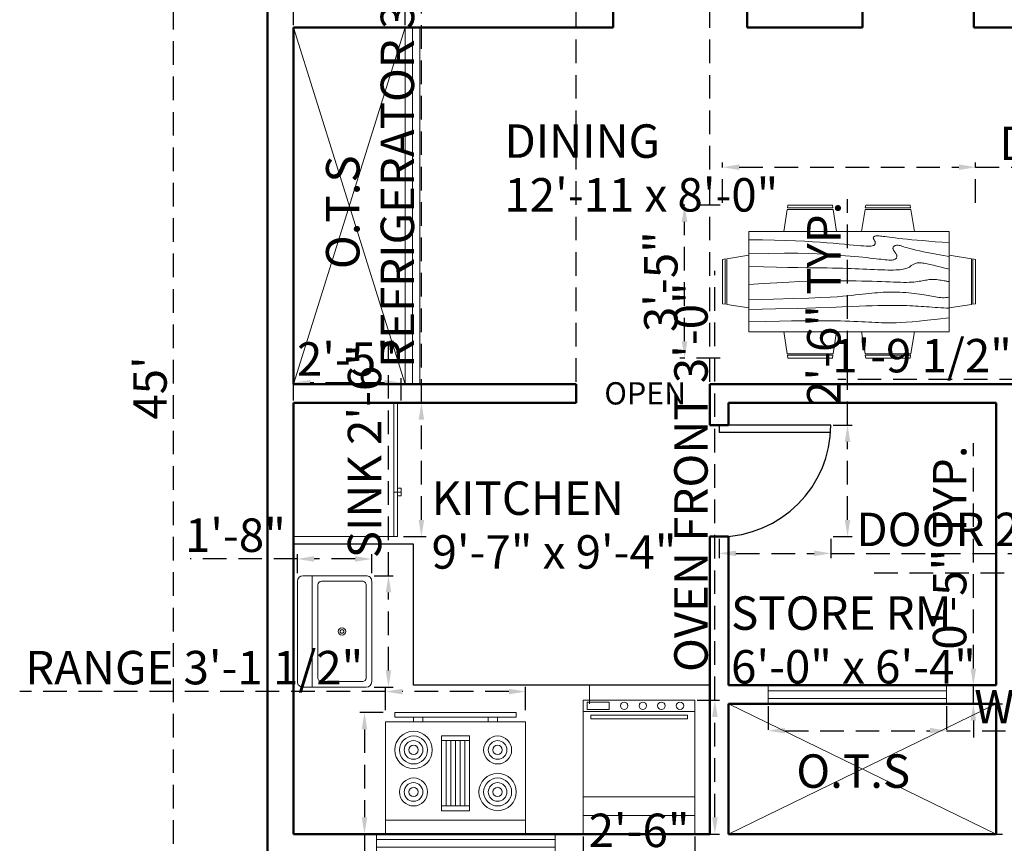
# Model space of a CAD drawing. Units: inches. Extents: x 3209 to 7144, y 1281 to 3076.
# Tile 2 of 5: x 3209 to 3474, y 1459 to 1680. Entities that reach past the tile are written whole.
import ezdxf

# ---------------------------------------------------------------- set-up
doc = ezdxf.new("R2010")
doc.units = ezdxf.units.IN
doc.linetypes.add('HIDDEN', pattern=[9.525, 6.35, -3.175])
for name, color, linetype, lineweight in [('A-ANNO-DIMS', 244, 'HIDDEN', 18), ('A-ANNO-TEXT', 7, 'Continuous', 18), ('A-AREA-IDEN', 7, 'Continuous', 25), ('A-DOOR', 4, 'Continuous', 25), ('A-EQPM', 9, 'Continuous', 18), ('A-FLOR-CASE', 8, 'Continuous', 25), ('A-FLOR-FIXT', 9, 'Continuous', 18), ('A-FLOR-OPEN', 8, 'Continuous', 13), ('A-FURN', 8, 'Continuous', 18), ('A-GLAZ', 4, 'Continuous', 18), ('A-WALL', 7, 'Continuous', 50)]:
    doc.layers.add(name, color=color, linetype=linetype, lineweight=lineweight)
doc.styles.get("Standard").update_dxf_attribs({"font": 'arial.ttf'})
doc.dimstyles.new('ISO-25', dxfattribs={"dimtxt": 9, "dimasz": 4.5, "dimexe": 1.25, "dimexo": 0.625, "dimtad": 1, "dimdec": 0, "dimlunit": 3, "dimtxsty": 'Standard', "dimcen": 2.5, "dimadec": 0, "dimazin": 0, "dimtfac": 1, "dimtdec": 0, "dimtmove": 0, "dimatfit": 3, "dimfxl": 1, "dimarcsym": 0})

# ---------------------------------------------------------------- blocks, each defined once
blk = doc.blocks.new('Dining Set - 36 x 72 in.')
for p, q in [((-22.2343, 26.00059), (-23.4847, 17.99762)), ((-22.2304, 26), (-5.7608, 26)), ((-22, 27.5), (-22.1562, 26.50042)), ((-5.8416, 26.5), (-22.1534, 26.5)), ((-22, 27.5), (-6, 27.5)), ((-5.8437, 26.49966), (-6, 27.5)), ((-4.5152, 17.99762), (-5.7655, 25.99926)), ((5.7657, 26.00059), (4.5153, 17.99762)), ((5.7696, 26), (22.2392, 26)), ((6, 27.5), (5.8438, 26.50042)), ((22.1584, 26.5), (5.8466, 26.5)), ((6, 27.5), (22, 27.5)), ((22.1563, 26.49966), (22, 27.5)), ((23.4848, 17.99762), (22.2345, 25.99926)), ((36, 18), (-36, 18)), ((-36, 18), (-36, -18)), ((36, -18), (36, 18)), ((-45.5, 8), (-44.5004, 8.15617)), ((-45.5, 8), (-45.5, -8)), ((-44.5, -8.15843), (-44.5, 8.15338)), ((-44.0006, 8.23428), (-35.9976, 9.48474)), ((-44, 8.23041), (-44, -8.23915)), ((44.0006, 8.23428), (35.9976, 9.48474)), ((44, 8.23041), (44, -8.23915)), ((44.5, -8.15843), (44.5, 8.15338)), ((45.5, 8), (44.5005, 8.15617)), ((45.5, 8), (45.5, -8)), ((-44.4997, -8.15631), (-45.5, -8)), ((-35.9976, -9.48476), (-43.9993, -8.2345)), ((35.9976, -9.48476), (43.9993, -8.2345)), ((44.4997, -8.15631), (45.5, -8)), ((-36, -18), (36, -18)), ((-22.2343, -26.0006), (-23.4847, -17.99762)), ((-4.5152, -17.99762), (-5.7655, -25.99928)), ((5.7657, -26.0006), (4.5153, -17.99762)), ((23.4848, -17.99762), (22.2345, -25.99928)), ((-22.2304, -26), (-5.7608, -26)), ((-22, -27.5), (-22.1562, -26.50044)), ((-5.8416, -26.5), (-22.1534, -26.5)), ((-22, -27.5), (-6, -27.5)), ((-5.8437, -26.49967), (-6, -27.5)), ((5.7696, -26), (22.2392, -26)), ((6, -27.5), (5.8438, -26.50044)), ((22.1584, -26.5), (5.8466, -26.5)), ((6, -27.5), (22, -27.5)), ((22.1563, -26.49967), (22, -27.5))]:
    blk.add_line(p, q)
for points in [[(-36, 15), (-31.1772, 14.97754), (-26.8079, 14.91406), (-22.8538, 14.81543), (-19.276, 14.6875), (-16.0362, 14.53613), (-13.0957, 14.36718), (-10.4159, 14.18652), (-7.9583, 14), (-5.6904, 13.81315), (-3.6035, 13.63021), (-1.6954, 13.45508), (0.0365, 13.29166), (1.5945, 13.14388), (2.9811, 13.01562), (4.1988, 12.9108), (5.25, 12.83333), (6.1393, 12.78613), (6.8802, 12.76823), (7.4883, 12.77767), (7.9792, 12.8125), (8.3685, 12.87077), (8.6719, 12.95052), (8.9049, 13.0498), (9.0833, 13.16666), (9.2205, 13.29899), (9.3216, 13.44401), (9.3895, 13.59879), (9.4271, 13.76041), (9.4373, 13.92594), (9.4232, 14.09245), (9.3875, 14.257), (9.3333, 14.41666), (9.2638, 14.56917), (9.1836, 14.71484), (9.0975, 14.85465), (9.0104, 14.98958), (8.9272, 15.1206), (8.8529, 15.2487), (8.7922, 15.37483), (8.75, 15.5), (8.7305, 15.62467), (8.7344, 15.74739), (8.7617, 15.86621), (8.8125, 15.97916), (8.8867, 16.08431), (8.9844, 16.17968), (9.1055, 16.26334), (9.25, 16.33333), (9.4189, 16.38802), (9.6172, 16.42708), (9.8506, 16.45052), (10.125, 16.45833), (10.4463, 16.45052), (10.8203, 16.42708), (11.2529, 16.38802), (11.75, 16.33333), (12.3184, 16.26318), (12.9694, 16.17838), (13.7151, 16.07991), (14.5677, 15.96875), (15.5395, 15.84586), (16.6426, 15.71224), (17.8893, 15.56884), (19.2917, 15.41666), (20.859, 15.25667), (22.5879, 15.08984), (24.4721, 14.91715), (26.5052, 14.73958), (28.6809, 14.5581), (30.9929, 14.3737), (33.4347, 14.18733), (36, 14)], [(-36, 10), (-28.9766, 10.14274), (-23.1725, 10.20442), (-18.4241, 10.19775), (-14.5677, 10.13541), (-11.4399, 10.03011), (-8.877, 9.89453), (-6.7154, 9.74137), (-4.7917, 9.58333), (-2.9698, 9.43082), (-1.2246, 9.28515), (0.4415, 9.14534), (2.026, 9.01041), (3.5266, 8.87939), (4.9408, 8.7513), (6.266, 8.62516), (7.5, 8.5), (8.6411, 8.37549), (9.6914, 8.2539), (10.6538, 8.13818), (11.5312, 8.03125), (12.3267, 7.93603), (13.043, 7.85547), (13.6831, 7.79248), (14.25, 7.75), (14.7471, 7.7303), (15.1797, 7.73307), (15.5537, 7.75732), (15.875, 7.80208), (16.1494, 7.86637), (16.3828, 7.94922), (16.5811, 8.04964), (16.75, 8.16666), (16.8944, 8.29915), (17.0143, 8.44531), (17.1089, 8.60319), (17.1771, 8.77083), (17.218, 8.94629), (17.2305, 9.1276), (17.2137, 9.31282), (17.1667, 9.5), (17.0895, 9.6875), (16.987, 9.875), (16.8649, 10.0625), (16.7292, 10.25), (16.5856, 10.4375), (16.4401, 10.625), (16.2985, 10.8125), (16.1667, 11), (16.05, 11.18733), (15.9518, 11.3737), (15.8752, 11.5581), (15.8229, 11.73958), (15.798, 11.91715), (15.8034, 12.08984), (15.842, 12.25667), (15.9167, 12.41666), (16.0295, 12.56836), (16.1784, 12.70833), (16.3605, 12.83268), (16.5729, 12.9375), (16.8127, 13.01888), (17.0768, 13.07291), (17.3625, 13.0957), (17.6667, 13.08333), (17.9894, 13.03312), (18.3418, 12.94726), (18.7382, 12.82918), (19.1927, 12.68229), (19.7195, 12.51001), (20.3327, 12.31575), (21.0465, 12.10294), (21.875, 11.875), (22.8357, 11.63354), (23.959, 11.37304), (25.2786, 11.08618), (26.8282, 10.76562), (28.6414, 10.40405), (30.752, 9.99414), (33.1936, 9.52856), (36, 9)], [(-36, 5.5), (-30.7157, 5.3348), (-26.069, 5.20963), (-21.9946, 5.11767), (-18.4271, 5.05208), (-15.3009, 5.00602), (-12.5508, 4.97265), (-10.1112, 4.94515), (-7.9167, 4.91666), (-5.909, 4.88167), (-4.0586, 4.83984), (-2.3429, 4.79215), (-0.7396, 4.73958), (0.7739, 4.6831), (2.22, 4.6237), (3.6213, 4.56233), (5, 4.5), (6.373, 4.43782), (7.7344, 4.3776), (9.0723, 4.32129), (10.375, 4.27083), (11.6309, 4.22819), (12.8281, 4.19531), (13.9551, 4.17415), (15, 4.16666), (15.954, 4.17448), (16.819, 4.19791), (17.6001, 4.23698), (18.3021, 4.29166), (18.9299, 4.36198), (19.4883, 4.44791), (19.9823, 4.54948), (20.4167, 4.66666), (20.7969, 4.79899), (21.1302, 4.94401), (21.4245, 5.09879), (21.6875, 5.26041), (21.9271, 5.42594), (22.1511, 5.59245), (22.3672, 5.757), (22.5834, 5.91666), (22.8065, 6.06868), (23.0404, 6.21093), (23.2879, 6.34147), (23.5521, 6.45833), (23.8358, 6.55957), (24.142, 6.64323), (24.4735, 6.70735), (24.8334, 6.75), (25.2235, 6.76969), (25.642, 6.76692), (26.0858, 6.74267), (26.5521, 6.69791), (27.0379, 6.63362), (27.5404, 6.55078), (28.0565, 6.45036), (28.5834, 6.33333), (29.1242, 6.19987), (29.7071, 6.04687), (30.3661, 5.87044), (31.1354, 5.66666), (32.0493, 5.43164), (33.142, 5.16146), (34.4475, 4.85221), (36, 4.5)], [(-36, -1), (-30.7915, -0.6591), (-26.0195, -0.38216), (-21.6519, -0.16284), (-17.6563, 0.00521), (-14.0005, 0.12833), (-10.6523, 0.21289), (-7.5796, 0.26522), (-4.75, 0.29166), (-2.134, 0.29793), (0.2878, 0.28711), (2.5317, 0.26163), (4.6146, 0.22396), (6.5529, 0.17651), (8.3633, 0.12174), (10.0623, 0.06209), (11.6667, 0), (13.1899, -0.06201), (14.6341, -0.1211), (15.9982, -0.17432), (17.2813, -0.21875), (18.4823, -0.25147), (19.6003, -0.26953), (20.6343, -0.27002), (21.5834, -0.25), (22.4481, -0.20768), (23.2357, -0.14584), (23.9549, -0.06836), (24.6146, 0.02083), (25.2235, 0.11784), (25.7904, 0.21875), (26.3241, 0.31966), (26.8334, 0.41666), (27.3265, 0.50618), (27.8099, 0.58593), (28.2894, 0.65397), (28.7709, 0.70833), (29.2601, 0.74707), (29.763, 0.76823), (30.2855, 0.76985), (30.8334, 0.75), (31.4088, 0.70784), (31.9994, 0.64713), (32.589, 0.57275), (33.1615, 0.48958), (33.7008, 0.4025), (34.1908, 0.3164), (34.6153, 0.23616), (34.9584, 0.16666), (35.2099, 0.11165), (35.3848, 0.07031), (35.504, 0.04069), (35.5886, 0.02083), (35.6594, 0.00879), (35.7377, 0.0026), (35.8442, 0.00032), (36, 0)], [(-36, -6.5), (-27.1843, -6.31267), (-20.084, -6.1263), (-14.469, -5.9419), (-10.1094, -5.76042), (-6.7752, -5.58285), (-4.2363, -5.41016), (-2.2629, -5.24333), (-0.625, -5.08334), (0.8708, -4.93099), (2.2715, -4.78646), (3.5872, -4.64974), (4.8281, -4.52084), (6.0046, -4.39974), (7.127, -4.28646), (8.2053, -4.18099), (9.25, -4.08334), (10.2705, -3.99382), (11.2734, -3.91407), (12.2647, -3.84603), (13.25, -3.79167), (14.2354, -3.75293), (15.2266, -3.73177), (16.2295, -3.73015), (17.25, -3.75), (18.2912, -3.79248), (19.3451, -3.85547), (20.4009, -3.93604), (21.4479, -4.03125), (22.4754, -4.13819), (23.4727, -4.25391), (24.4289, -4.37549), (25.3334, -4.5), (26.1785, -4.62492), (26.9694, -4.74935), (27.7145, -4.87281), (28.4219, -4.99479), (29.1, -5.11483), (29.7572, -5.23242), (30.4016, -5.34709), (31.0417, -5.45834), (31.6837, -5.56437), (32.3262, -5.65821), (32.9658, -5.73153), (33.599, -5.77604), (34.2224, -5.78345), (34.8327, -5.74545), (35.4264, -5.65373), (36, -5.5)], [(-36, -10), (-26.4022, -9.81299), (-18.4675, -9.62891), (-11.9839, -9.45069), (-6.7396, -9.28125), (-2.5226, -9.12354), (0.8789, -8.98047), (3.6769, -8.85498), (6.0833, -8.75), (8.2767, -8.66765), (10.3021, -8.60677), (12.1712, -8.56543), (13.8958, -8.54167), (15.4876, -8.53353), (16.9583, -8.53907), (18.3197, -8.55632), (19.5834, -8.58334), (20.7616, -8.61841), (21.8685, -8.66081), (22.9188, -8.71004), (23.9271, -8.76563), (24.9081, -8.82707), (25.8763, -8.89388), (26.8465, -8.96558), (27.8334, -9.04167), (28.8474, -9.12118), (29.8828, -9.20117), (30.93, -9.27824), (31.9792, -9.34896), (33.0205, -9.40991), (34.0443, -9.45768), (35.0407, -9.48885), (36, -9.5)], [(-36, -14.5), (-30.0881, -14.33513), (-25.0332, -14.21224), (-20.7312, -14.12647), (-17.0781, -14.07292), (-13.97, -14.04671), (-11.3027, -14.04297), (-8.9724, -14.05681), (-6.875, -14.08334), (-4.9224, -14.11833), (-3.0905, -14.16016), (-1.3709, -14.20785), (0.2448, -14.26042), (1.7647, -14.3169), (3.1973, -14.3763), (4.5507, -14.43767), (5.8333, -14.5), (7.0554, -14.5621), (8.235, -14.62175), (9.3922, -14.67652), (10.5469, -14.72396), (11.7192, -14.76164), (12.929, -14.78711), (14.1965, -14.79794), (15.5417, -14.79167), (16.9933, -14.76424), (18.6152, -14.70508), (20.4804, -14.60197), (22.6615, -14.44271), (25.2312, -14.21509), (28.2624, -13.9069), (31.8277, -13.50594), (36, -13)]]:
    blk.add_lwpolyline(points)
blk = doc.blocks.new('Range-Oven - 30 in front')
for p, q in [((0, 33.00005), (30, 33.00005)), ((30, 10), (0, 10)), ((0, 5), (30, 5))]:
    blk.add_line(p, q)
for points in [[(0, 0), (0, 36.00005), (30, 36.00005), (30, 0)], [(1, 33.50005), (1, 35.50005), (7, 35.50005), (7, 33.50005)], [(2, 31.00005), (2, 32.00005), (28, 32.00005), (28, 31.00005)]]:
    blk.add_lwpolyline(points, close=True)
for centre in [(11, 34.50005), (16, 34.50005), (21, 34.50005), (26, 34.50005)]:
    blk.add_circle(centre, 1)
blk = doc.blocks.new('Sink-single - 30 in top')
blk.add_line((-15, -3.999996), (15, -3.999996))
for points in [[(-13.5, 0), (13.5, 0)], [(-15, -18.499996), (-15, -1.5)], [(15, -1.5), (15, -18.499996)], [(-13.5, -17.499996), (-13.5, -6.499996)], [(-12.5, -5.499996), (12.5, -5.499996)], [(13.5, -6.499996), (13.5, -17.499996)], [(12.5, -18.499996), (-12.5, -18.499996)], [(13.5, -19.999996), (-13.5, -19.999996)]]:
    blk.add_lwpolyline(points)
for radius in [1, 0.5]:
    blk.add_circle((0, -11.999996), radius)
for centre, radius, start, end in [((-13.5, -1.5), 1.5, 90, 180), ((13.5, -1.5), 1.5, 0, 90), ((-12.5, -6.499996), 1, 90, 180), ((12.5, -6.499996), 1, 0, 90), ((-13.5, -18.499996), 1.5, 180, 270), ((-12.5, -17.499996), 1, 180, 270), ((12.5, -17.499996), 1, 270, 0), ((13.5, -18.499996), 1.5, 270, 0)]:
    blk.add_arc(centre, radius, start, end)
blk = doc.blocks.new('Refrigerator-2 door - 36 in top')
for p, q in [((0, -26.999999), (36, -26.999999)), ((11, -27.999999), (11, -28.999999)), ((11, -28.999999), (13, -28.999999)), ((12, -26.999999), (12, -28.999999)), ((13, -28.999999), (13, -27.999999))]:
    blk.add_line(p, q)
blk.add_lwpolyline([(0, -27.999999), (0, 0), (36, 0), (36, -27.999999)], close=True)
blk = doc.blocks.new('Range-Oven - 30 in top')
for p, q in [((0, -3), (30, -3)), ((12, -6), (18, -6)), ((13, -20), (13, -6)), ((14, -6), (14, -20)), ((15, -20), (15, -6)), ((16, -6), (16, -20)), ((17, -20), (17, -6)), ((18, -20), (12, -20)), ((6, -24), (6, -25)), ((8, -25), (8, -24)), ((22, -25), (22, -24)), ((24, -24), (24, -25))]:
    blk.add_line(p, q)
for points in [[(0, -24), (0, 0), (30, 0), (30, -24)], [(12, -21), (12, -5), (18, -5), (18, -21)], [(2, -26), (2, -25), (28, -25), (28, -26)]]:
    blk.add_lwpolyline(points, close=True)
for centre, radius in [((6, -9), 4), ((6, -9), 3), ((24, -9), 3), ((6, -9), 2), ((6, -9), 1), ((24, -9), 2), ((24, -9), 1), ((24, -18), 4), ((6, -18), 3), ((6, -18), 2), ((24, -18), 3), ((24, -18), 2), ((6, -18), 1), ((24, -18), 1)]:
    blk.add_circle(centre, radius)
blk = doc.blocks.new('*D15')
at = {"layer": 'A-ANNO-DIMS', "color": 0, "lineweight": -2, "transparency": 16777216}
for p, q in [((3275.31, 1851.27), (3249.46, 1851.27)), ((3250.71, 1315.77), (3250.71, 1846.77)), ((3275.31, 1311.27), (3249.46, 1311.27))]:
    blk.add_line(p, q, dxfattribs=at)
at = {"layer": 'A-ANNO-DIMS', "color": 0, "transparency": 16777216}
for points in [[(3249.96, 1846.77), (3251.46, 1846.77), (3250.71, 1851.27)], [(3249.96, 1315.77), (3251.46, 1315.77), (3250.71, 1311.27)]]:
    blk.add_solid(points, dxfattribs=at)
at = {"layer": 'Defpoints', "color": 0, "transparency": 16777216}
for p in [(3250.71, 1851.27), (3275.94, 1851.27), (3275.94, 1311.27)]:
    blk.add_point(p, dxfattribs=at)
at = {"layer": 'A-ANNO-DIMS', "color": 0, "transparency": 16777216, "insert": (3245.51, 1581.27), "char_height": 9, "attachment_point": 5, "rotation": 90}
blk.add_mtext("45'", dxfattribs=at)
blk = doc.blocks.new('DOOR-SWING-30IN')
for p, q in [((30, 30), (0, 30)), ((0, 30), (0, 28)), ((30, 28), (0, 28))]:
    blk.add_line(p, q)
blk.add_arc((0, 30), 30, 270, 0)
blk = doc.blocks.new('WINDOW-48IN-WALL5')
for p, q in [((0, 5), (0, 0)), ((0, 3.5), (48, 3.5)), ((48, 5), (48, 0)), ((0, 1.5), (48, 1.5))]:
    blk.add_line(p, q)
blk = doc.blocks.new('*D42')
at = {"layer": 'A-ANNO-DIMS', "color": 0, "lineweight": -2, "transparency": 16777216}
for p, q in [((3397.44, 1540.64), (3397.44, 1535.52)), ((3427.44, 1540.64), (3427.44, 1535.52)), ((3401.94, 1536.77), (3422.94, 1536.77)), ((3427.44, 1536.77), (3528.81, 1536.77))]:
    blk.add_line(p, q, dxfattribs=at)
at = {"layer": 'A-ANNO-DIMS', "color": 0, "transparency": 16777216}
for points in [[(3401.94, 1537.52), (3401.94, 1536.02), (3397.44, 1536.77)], [(3422.94, 1537.52), (3422.94, 1536.02), (3427.44, 1536.77)]]:
    blk.add_solid(points, dxfattribs=at)
at = {"layer": 'Defpoints', "color": 0, "transparency": 16777216}
for p in [(3397.44, 1541.27), (3427.44, 1541.27), (3427.44, 1536.77)]:
    blk.add_point(p, dxfattribs=at)
at = {"layer": 'A-ANNO-DIMS', "color": 0, "transparency": 16777216, "insert": (3480.37, 1542.05), "char_height": 9, "attachment_point": 5}
blk.add_mtext('DOOR 2\'-6" TYP.', dxfattribs=at)
blk = doc.blocks.new('*D43')
at = {"layer": 'A-ANNO-DIMS', "color": 0, "lineweight": -2, "transparency": 16777216}
for p, q in [((3431.94, 1571.27), (3431.94, 1632.03)), ((3428.06, 1571.27), (3433.19, 1571.27)), ((3431.94, 1545.77), (3431.94, 1566.77)), ((3428.06, 1541.27), (3433.19, 1541.27))]:
    blk.add_line(p, q, dxfattribs=at)
at = {"layer": 'A-ANNO-DIMS', "color": 0, "transparency": 16777216}
for points in [[(3431.19, 1566.77), (3432.69, 1566.77), (3431.94, 1571.27)], [(3431.19, 1545.77), (3432.69, 1545.77), (3431.94, 1541.27)]]:
    blk.add_solid(points, dxfattribs=at)
at = {"layer": 'Defpoints', "color": 0, "transparency": 16777216}
for p in [(3427.44, 1571.27), (3431.94, 1571.27), (3427.44, 1541.27)]:
    blk.add_point(p, dxfattribs=at)
at = {"layer": 'A-ANNO-DIMS', "color": 0, "transparency": 16777216, "insert": (3426.72, 1603.9), "char_height": 9, "attachment_point": 5, "rotation": 90}
blk.add_mtext('2\'-6" TYP.', dxfattribs=at)
blk = doc.blocks.new('*D46')
at = {"layer": 'A-ANNO-DIMS', "color": 0, "lineweight": -2, "transparency": 16777216}
for p, q in [((3410.58, 1495.64), (3410.58, 1487.82)), ((3458.58, 1495.64), (3458.58, 1487.82)), ((3415.08, 1489.07), (3454.08, 1489.07)), ((3458.58, 1489.07), (3578.22, 1489.07))]:
    blk.add_line(p, q, dxfattribs=at)
at = {"layer": 'A-ANNO-DIMS', "color": 0, "transparency": 16777216}
for points in [[(3415.08, 1489.82), (3415.08, 1488.32), (3410.58, 1489.07)], [(3454.08, 1489.82), (3454.08, 1488.32), (3458.58, 1489.07)]]:
    blk.add_solid(points, dxfattribs=at)
at = {"layer": 'Defpoints', "color": 0, "transparency": 16777216}
for p in [(3410.58, 1496.27), (3458.58, 1496.27), (3458.58, 1489.07)]:
    blk.add_point(p, dxfattribs=at)
at = {"layer": 'A-ANNO-DIMS', "color": 0, "transparency": 16777216, "insert": (3520.65, 1494.35), "char_height": 9, "attachment_point": 5}
blk.add_mtext('WINDOW 4\'-0" TYP.', dxfattribs=at)
blk = doc.blocks.new('*D47')
at = {"layer": 'A-ANNO-DIMS', "color": 0, "lineweight": -2, "transparency": 16777216}
for p, q in [((3465.78, 1505.77), (3465.78, 1566.38)), ((3459.21, 1501.27), (3467.03, 1501.27)), ((3465.78, 1496.27), (3465.78, 1501.27)), ((3459.21, 1496.27), (3467.03, 1496.27)), ((3465.78, 1491.77), (3465.78, 1487.27))]:
    blk.add_line(p, q, dxfattribs=at)
at = {"layer": 'A-ANNO-DIMS', "color": 0, "transparency": 16777216}
for points in [[(3465.03, 1505.77), (3466.53, 1505.77), (3465.78, 1501.27)], [(3465.03, 1491.77), (3466.53, 1491.77), (3465.78, 1496.27)]]:
    blk.add_solid(points, dxfattribs=at)
at = {"layer": 'Defpoints', "color": 0, "transparency": 16777216}
for p in [(3458.58, 1501.27), (3465.78, 1501.27), (3458.58, 1496.27)]:
    blk.add_point(p, dxfattribs=at)
at = {"layer": 'A-ANNO-DIMS', "color": 0, "transparency": 16777216, "insert": (3460.56, 1538.32), "char_height": 9, "attachment_point": 5, "rotation": 90}
blk.add_mtext('0\'-5" TYP.', dxfattribs=at)
blk = doc.blocks.new('*D52')
at = {"layer": 'A-ANNO-DIMS', "color": 0, "lineweight": -2, "transparency": 16777216}
for p, q in [((3398.32, 1631.06), (3398.32, 1641.9)), ((3466.38, 1631.06), (3466.38, 1641.9)), ((3402.82, 1640.65), (3461.88, 1640.65)), ((3466.38, 1640.65), (3571.05, 1640.65))]:
    blk.add_line(p, q, dxfattribs=at)
at = {"layer": 'A-ANNO-DIMS', "color": 0, "transparency": 16777216}
for points in [[(3402.82, 1641.4), (3402.82, 1639.9), (3398.32, 1640.65)], [(3461.88, 1641.4), (3461.88, 1639.9), (3466.38, 1640.65)]]:
    blk.add_solid(points, dxfattribs=at)
at = {"layer": 'Defpoints', "color": 0, "transparency": 16777216}
for p in [(3466.38, 1640.65), (3398.32, 1630.44), (3466.38, 1630.44)]:
    blk.add_point(p, dxfattribs=at)
at = {"layer": 'A-ANNO-DIMS', "color": 0, "transparency": 16777216, "insert": (3520.96, 1645.92), "char_height": 9, "attachment_point": 5}
blk.add_mtext('DINING SET 5\'-8"', dxfattribs=at)
blk = doc.blocks.new('*D53')
at = {"layer": 'A-ANNO-DIMS', "color": 0, "lineweight": -2, "transparency": 16777216}
for p, q in [((3397.7, 1630.44), (3386.86, 1630.44)), ((3388.11, 1593.81), (3388.11, 1625.94)), ((3397.7, 1589.31), (3386.86, 1589.31))]:
    blk.add_line(p, q, dxfattribs=at)
at = {"layer": 'A-ANNO-DIMS', "color": 0, "transparency": 16777216}
for points in [[(3387.36, 1625.94), (3388.86, 1625.94), (3388.11, 1630.44)], [(3387.36, 1593.81), (3388.86, 1593.81), (3388.11, 1589.31)]]:
    blk.add_solid(points, dxfattribs=at)
at = {"layer": 'Defpoints', "color": 0, "transparency": 16777216}
for p in [(3388.11, 1630.44), (3398.32, 1630.44), (3398.32, 1589.31)]:
    blk.add_point(p, dxfattribs=at)
at = {"layer": 'A-ANNO-DIMS', "color": 0, "transparency": 16777216, "insert": (3382.89, 1609.87), "char_height": 9, "attachment_point": 5, "rotation": 90}
blk.add_mtext('3\'-5"', dxfattribs=at)
blk = doc.blocks.new('*D55')
at = {"layer": 'A-ANNO-DIMS', "color": 0, "lineweight": -2, "transparency": 16777216}
for p, q in [((3479.12, 1583.5), (3429.33, 1583.5)), ((3479.12, 1575.13), (3479.12, 1584.75)), ((3495.96, 1583.5), (3483.62, 1583.5)), ((3500.46, 1575.13), (3500.46, 1584.75))]:
    blk.add_line(p, q, dxfattribs=at)
at = {"layer": 'A-ANNO-DIMS', "color": 0, "transparency": 16777216}
for points in [[(3483.62, 1584.25), (3483.62, 1582.75), (3479.12, 1583.5)], [(3495.96, 1584.25), (3495.96, 1582.75), (3500.46, 1583.5)]]:
    blk.add_solid(points, dxfattribs=at)
at = {"layer": 'Defpoints', "color": 0, "transparency": 16777216}
for p in [(3479.12, 1583.5), (3479.12, 1574.5), (3500.46, 1574.5)]:
    blk.add_point(p, dxfattribs=at)
at = {"layer": 'A-ANNO-DIMS', "color": 0, "transparency": 16777216, "insert": (3451.97, 1588.78), "char_height": 9, "attachment_point": 5}
blk.add_mtext('1\'-9 1/2"', dxfattribs=at)
blk = doc.blocks.new('*D56')
at = {"layer": 'A-ANNO-DIMS', "color": 0, "lineweight": -2, "transparency": 16777216}
for p, q in [((3396.28, 1497.27), (3396.28, 1612.78)), ((3391.51, 1497.27), (3397.53, 1497.27)), ((3396.28, 1465.77), (3396.28, 1492.77)), ((3391.51, 1461.27), (3397.53, 1461.27))]:
    blk.add_line(p, q, dxfattribs=at)
at = {"layer": 'A-ANNO-DIMS', "color": 0, "transparency": 16777216}
for points in [[(3395.53, 1492.77), (3397.03, 1492.77), (3396.28, 1497.27)], [(3395.53, 1465.77), (3397.03, 1465.77), (3396.28, 1461.27)]]:
    blk.add_solid(points, dxfattribs=at)
at = {"layer": 'Defpoints', "color": 0, "transparency": 16777216}
for p in [(3390.88, 1497.27), (3396.28, 1497.27), (3390.88, 1461.27)]:
    blk.add_point(p, dxfattribs=at)
at = {"layer": 'A-ANNO-DIMS', "color": 0, "transparency": 16777216, "insert": (3391, 1557.27), "char_height": 9, "attachment_point": 5, "rotation": 90}
blk.add_mtext('OVEN FRONT 3\'-0"', dxfattribs=at)
blk = doc.blocks.new('*D57')
at = {"layer": 'A-ANNO-DIMS', "color": 0, "lineweight": -2, "transparency": 16777216}
for p, q in [((3360.88, 1460.64), (3360.88, 1454.62)), ((3390.88, 1460.64), (3390.88, 1454.62)), ((3365.38, 1455.87), (3386.38, 1455.87))]:
    blk.add_line(p, q, dxfattribs=at)
at = {"layer": 'A-ANNO-DIMS', "color": 0, "transparency": 16777216}
for points in [[(3365.38, 1456.62), (3365.38, 1455.12), (3360.88, 1455.87)], [(3386.38, 1456.62), (3386.38, 1455.12), (3390.88, 1455.87)]]:
    blk.add_solid(points, dxfattribs=at)
at = {"layer": 'Defpoints', "color": 0, "transparency": 16777216}
for p in [(3360.88, 1461.27), (3390.88, 1461.27), (3390.88, 1455.87)]:
    blk.add_point(p, dxfattribs=at)
at = {"layer": 'A-ANNO-DIMS', "color": 0, "transparency": 16777216, "insert": (3375.88, 1461.09), "char_height": 9, "attachment_point": 5}
blk.add_mtext('2\'-6"', dxfattribs=at)
blk = doc.blocks.new('*D58')
at = {"layer": 'A-ANNO-DIMS', "color": 0, "lineweight": -2, "transparency": 16777216}
for p, q in [((3308.49, 1530.77), (3308.49, 1593.24)), ((3304.61, 1530.77), (3309.74, 1530.77)), ((3308.49, 1505.27), (3308.49, 1526.27)), ((3304.61, 1500.77), (3309.74, 1500.77))]:
    blk.add_line(p, q, dxfattribs=at)
at = {"layer": 'A-ANNO-DIMS', "color": 0, "transparency": 16777216}
for points in [[(3307.74, 1526.27), (3309.24, 1526.27), (3308.49, 1530.77)], [(3307.74, 1505.27), (3309.24, 1505.27), (3308.49, 1500.77)]]:
    blk.add_solid(points, dxfattribs=at)
at = {"layer": 'Defpoints', "color": 0, "transparency": 16777216}
for p in [(3303.99, 1530.77), (3308.49, 1530.77), (3303.99, 1500.77)]:
    blk.add_point(p, dxfattribs=at)
at = {"layer": 'A-ANNO-DIMS', "color": 0, "transparency": 16777216, "insert": (3303.21, 1564.26), "char_height": 9, "attachment_point": 5, "rotation": 90}
blk.add_mtext('SINK 2\'-6"', dxfattribs=at)
blk = doc.blocks.new('*D59')
at = {"layer": 'A-ANNO-DIMS', "color": 0, "lineweight": -2, "transparency": 16777216}
for p, q in [((3283.99, 1531.4), (3283.99, 1536.52)), ((3303.99, 1531.4), (3303.99, 1536.52)), ((3283.99, 1535.27), (3255.16, 1535.27)), ((3299.49, 1535.27), (3288.49, 1535.27))]:
    blk.add_line(p, q, dxfattribs=at)
at = {"layer": 'A-ANNO-DIMS', "color": 0, "transparency": 16777216}
for points in [[(3288.49, 1536.02), (3288.49, 1534.52), (3283.99, 1535.27)], [(3299.49, 1536.02), (3299.49, 1534.52), (3303.99, 1535.27)]]:
    blk.add_solid(points, dxfattribs=at)
at = {"layer": 'Defpoints', "color": 0, "transparency": 16777216}
for p in [(3283.99, 1535.27), (3283.99, 1530.77), (3303.99, 1530.77)]:
    blk.add_point(p, dxfattribs=at)
at = {"layer": 'A-ANNO-DIMS', "color": 0, "transparency": 16777216, "insert": (3267.32, 1540.49), "char_height": 9, "attachment_point": 5}
blk.add_mtext('1\'-8"', dxfattribs=at)
blk = doc.blocks.new('*D60')
at = {"layer": 'A-ANNO-DIMS', "color": 0, "lineweight": -2, "transparency": 16777216}
for p, q in [((3317.34, 1577.27), (3317.34, 1709.86)), ((3312.56, 1577.27), (3318.59, 1577.27)), ((3317.34, 1545.77), (3317.34, 1572.77)), ((3312.56, 1541.27), (3318.59, 1541.27))]:
    blk.add_line(p, q, dxfattribs=at)
at = {"layer": 'A-ANNO-DIMS', "color": 0, "transparency": 16777216}
for points in [[(3316.59, 1572.77), (3318.09, 1572.77), (3317.34, 1577.27)], [(3316.59, 1545.77), (3318.09, 1545.77), (3317.34, 1541.27)]]:
    blk.add_solid(points, dxfattribs=at)
at = {"layer": 'Defpoints', "color": 0, "transparency": 16777216}
for p in [(3311.94, 1577.27), (3317.34, 1577.27), (3311.94, 1541.27)]:
    blk.add_point(p, dxfattribs=at)
at = {"layer": 'A-ANNO-DIMS', "color": 0, "transparency": 16777216, "insert": (3312.05, 1645.82), "char_height": 9, "attachment_point": 5, "rotation": 90}
blk.add_mtext('REFRIGERATOR 3\'-0"', dxfattribs=at)
blk = doc.blocks.new('*D61')
at = {"layer": 'A-ANNO-DIMS', "color": 0, "lineweight": -2, "transparency": 16777216}
for p, q in [((3282.94, 1577.89), (3282.94, 1583.92)), ((3311.94, 1577.89), (3311.94, 1583.92)), ((3307.44, 1582.67), (3287.44, 1582.67))]:
    blk.add_line(p, q, dxfattribs=at)
at = {"layer": 'A-ANNO-DIMS', "color": 0, "transparency": 16777216}
for points in [[(3287.44, 1583.42), (3287.44, 1581.92), (3282.94, 1582.67)], [(3307.44, 1583.42), (3307.44, 1581.92), (3311.94, 1582.67)]]:
    blk.add_solid(points, dxfattribs=at)
at = {"layer": 'Defpoints', "color": 0, "transparency": 16777216}
for p in [(3282.94, 1582.67), (3282.94, 1577.27), (3311.94, 1577.27)]:
    blk.add_point(p, dxfattribs=at)
at = {"layer": 'A-ANNO-DIMS', "color": 0, "transparency": 16777216, "insert": (3297.44, 1587.89), "char_height": 9, "attachment_point": 5}
blk.add_mtext('2\'-5"', dxfattribs=at)
blk = doc.blocks.new('*D62')
at = {"layer": 'A-ANNO-DIMS', "color": 0, "lineweight": -2, "transparency": 16777216}
for p, q in [((3307.69, 1499.59), (3209.31, 1499.59)), ((3307.69, 1494.56), (3307.69, 1500.84)), ((3340.88, 1499.59), (3312.19, 1499.59)), ((3345.38, 1494.56), (3345.38, 1500.84))]:
    blk.add_line(p, q, dxfattribs=at)
at = {"layer": 'A-ANNO-DIMS', "color": 0, "transparency": 16777216}
for points in [[(3312.19, 1500.34), (3312.19, 1498.84), (3307.69, 1499.59)], [(3340.88, 1500.34), (3340.88, 1498.84), (3345.38, 1499.59)]]:
    blk.add_solid(points, dxfattribs=at)
at = {"layer": 'Defpoints', "color": 0, "transparency": 16777216}
for p in [(3307.69, 1499.59), (3307.69, 1493.93), (3345.38, 1493.93)]:
    blk.add_point(p, dxfattribs=at)
at = {"layer": 'A-ANNO-DIMS', "color": 0, "transparency": 16777216, "insert": (3256.25, 1504.87), "char_height": 9, "attachment_point": 5}
blk.add_mtext('RANGE 3\'-1 1/2"', dxfattribs=at)
blk = doc.blocks.new('*D63')
at = {"layer": 'A-ANNO-DIMS', "color": 0, "lineweight": -2, "transparency": 16777216}
for p, q in [((3307.07, 1493.93), (3300.79, 1493.93)), ((3302.04, 1489.43), (3302.04, 1465.77)), ((3307.07, 1461.27), (3300.79, 1461.27)), ((3302.04, 1461.27), (3302.04, 1410.47))]:
    blk.add_line(p, q, dxfattribs=at)
at = {"layer": 'A-ANNO-DIMS', "color": 0, "transparency": 16777216}
for points in [[(3301.29, 1489.43), (3302.79, 1489.43), (3302.04, 1493.93)], [(3301.29, 1465.77), (3302.79, 1465.77), (3302.04, 1461.27)]]:
    blk.add_solid(points, dxfattribs=at)
at = {"layer": 'Defpoints', "color": 0, "transparency": 16777216}
for p in [(3307.69, 1493.93), (3302.04, 1461.27), (3307.69, 1461.27)]:
    blk.add_point(p, dxfattribs=at)
at = {"layer": 'A-ANNO-DIMS', "color": 0, "transparency": 16777216, "insert": (3296.76, 1433.62), "char_height": 9, "attachment_point": 5, "rotation": 90}
blk.add_mtext('2\'-8 1/2"', dxfattribs=at)
blk = doc.blocks.new('*D73')
at = {"layer": 'A-ANNO-DIMS', "color": 0, "lineweight": -2, "transparency": 16777216}
for p, q in [((3400.56, 1496.27), (3665.83, 1496.27)), ((3664.58, 1465.77), (3664.58, 1491.77)), ((3400.56, 1461.27), (3665.83, 1461.27))]:
    blk.add_line(p, q, dxfattribs=at)
at = {"layer": 'A-ANNO-DIMS', "color": 0, "transparency": 16777216}
for points in [[(3663.83, 1491.77), (3665.33, 1491.77), (3664.58, 1496.27)], [(3663.83, 1465.77), (3665.33, 1465.77), (3664.58, 1461.27)]]:
    blk.add_solid(points, dxfattribs=at)
at = {"layer": 'Defpoints', "color": 0, "transparency": 16777216}
for p in [(3399.94, 1496.27), (3664.58, 1496.27), (3399.94, 1461.27)]:
    blk.add_point(p, dxfattribs=at)
at = {"layer": 'A-ANNO-DIMS', "color": 0, "transparency": 16777216, "insert": (3659.44, 1478.77), "char_height": 9, "attachment_point": 5, "rotation": 90}
blk.add_mtext('2\'-11"', dxfattribs=at)
blk = doc.blocks.new('*D74')
at = {"layer": 'A-ANNO-DIMS', "color": 0, "lineweight": -2, "transparency": 16777216}
for p, q in [((3282.94, 1678.89), (3282.94, 1881.16)), ((3312.94, 1678.89), (3312.94, 1881.16)), ((3287.44, 1879.91), (3308.44, 1879.91))]:
    blk.add_line(p, q, dxfattribs=at)
at = {"layer": 'A-ANNO-DIMS', "color": 0, "transparency": 16777216}
for points in [[(3287.44, 1880.66), (3287.44, 1879.16), (3282.94, 1879.91)], [(3308.44, 1880.66), (3308.44, 1879.16), (3312.94, 1879.91)]]:
    blk.add_solid(points, dxfattribs=at)
at = {"layer": 'Defpoints', "color": 0, "transparency": 16777216}
for p in [(3312.94, 1879.91), (3282.94, 1678.27), (3312.94, 1678.27)]:
    blk.add_point(p, dxfattribs=at)
at = {"layer": 'A-ANNO-DIMS', "color": 0, "transparency": 16777216, "insert": (3297.94, 1885.14), "char_height": 9, "attachment_point": 5}
blk.add_mtext('2\'-6"', dxfattribs=at)
blk = doc.blocks.new('*D75')
at = {"layer": 'A-ANNO-DIMS', "color": 0, "lineweight": -2, "transparency": 16777216}
for p, q in [((3358.94, 1582.89), (3358.94, 1881.16)), ((3394.94, 1582.89), (3394.94, 1881.16)), ((3363.44, 1879.91), (3390.44, 1879.91))]:
    blk.add_line(p, q, dxfattribs=at)
at = {"layer": 'A-ANNO-DIMS', "color": 0, "transparency": 16777216}
for points in [[(3363.44, 1880.66), (3363.44, 1879.16), (3358.94, 1879.91)], [(3390.44, 1880.66), (3390.44, 1879.16), (3394.94, 1879.91)]]:
    blk.add_solid(points, dxfattribs=at)
at = {"layer": 'Defpoints', "color": 0, "transparency": 16777216}
for p in [(3394.94, 1879.91), (3358.94, 1582.27), (3394.94, 1582.27)]:
    blk.add_point(p, dxfattribs=at)
at = {"layer": 'A-ANNO-DIMS', "color": 0, "transparency": 16777216, "insert": (3376.94, 1885.14), "char_height": 9, "attachment_point": 5}
blk.add_mtext('3\'-0"', dxfattribs=at)
blk = doc.blocks.new('*D83')
at = {"layer": 'A-ANNO-DIMS', "color": 0, "lineweight": -2, "transparency": 16777216}
for p, q in [((3439.12, 1531.5), (3500.12, 1531.5)), ((3553.62, 1531.5), (3504.62, 1531.5))]:
    blk.add_line(p, q, dxfattribs=at)
at = {"layer": 'A-ANNO-DIMS', "color": 0, "transparency": 16777216}
blk.add_solid([(3504.62, 1532.25), (3504.62, 1530.75), (3500.12, 1531.5)], dxfattribs=at)
at = {"layer": 'Defpoints', "color": 0, "transparency": 16777216}
for p in [(3439.12, 1531.5), (3500.12, 1531.5)]:
    blk.add_point(p, dxfattribs=at)
at = {"layer": 'A-ANNO-DIMS', "color": 0, "transparency": 16777216, "insert": (3536.72, 1536.72), "char_height": 9, "attachment_point": 5, "rotation": 0.0002}
blk.add_mtext('R5\'-1"', dxfattribs=at)

msp = doc.modelspace()

# ---------------------------------------------------------------- linework, layer by layer
at = {"layer": 'A-FLOR-CASE'}
for p, q in [((3315.25, 1539.27), (3282.94, 1539.27)), ((3315.25, 1501.27), (3315.25, 1539.27)), ((3394.94, 1501.27), (3315.25, 1501.27))]:
    msp.add_line(p, q, dxfattribs=at)
at = {"layer": 'A-FLOR-OPEN'}
for p, q in [((3282.94, 1678.27), (3312.94, 1582.27)), ((3282.94, 1582.27), (3312.94, 1678.27)), ((3399.94, 1496.27), (3471.94, 1461.27)), ((3471.94, 1496.27), (3399.94, 1461.27))]:
    msp.add_line(p, q, dxfattribs=at)
at = {"layer": 'A-GLAZ'}
for p, q in [((3312.94, 1582.27), (3312.94, 1678.27)), ((3314.94, 1582.27), (3314.94, 1678.27)), ((3316.94, 1582.27), (3316.94, 1678.27)), ((3362.58, 1501.27), (3362.58, 1496.27))]:
    msp.add_line(p, q, dxfattribs=at)
at = {"layer": 'A-WALL'}
for p, q in [((3275.94, 1311.27), (3275.94, 1851.27)), ((3368.94, 1678.27), (3368.94, 1683.27)), ((3404.94, 1678.27), (3404.94, 1683.27)), ((3435.94, 1683.27), (3435.94, 1678.27)), ((3465.94, 1683.27), (3465.94, 1678.27)), ((3282.94, 1678.27), (3368.94, 1678.27)), ((3282.94, 1582.27), (3282.94, 1678.27)), ((3404.94, 1678.27), (3415.94, 1678.27)), ((3415.94, 1678.27), (3435.94, 1678.27)), ((3465.94, 1678.27), (3482.94, 1678.27)), ((3282.94, 1582.27), (3358.94, 1582.27)), ((3358.94, 1582.27), (3358.94, 1577.27)), ((3394.94, 1582.27), (3394.94, 1571.27)), ((3394.94, 1582.27), (3476.94, 1582.27)), ((3282.94, 1577.27), (3358.94, 1577.27)), ((3282.94, 1461.27), (3282.94, 1577.27)), ((3399.94, 1577.27), (3399.94, 1571.27)), ((3399.94, 1577.27), (3471.94, 1577.27)), ((3471.94, 1577.27), (3471.94, 1501.27)), ((3394.94, 1571.27), (3399.94, 1571.27)), ((3394.94, 1541.27), (3399.94, 1541.27)), ((3394.94, 1541.27), (3394.94, 1461.27)), ((3399.94, 1541.27), (3399.94, 1501.27)), ((3399.94, 1501.27), (3471.94, 1501.27)), ((3399.94, 1496.27), (3471.94, 1496.27)), ((3399.94, 1496.27), (3399.94, 1461.27)), ((3471.94, 1496.27), (3471.94, 1461.27)), ((3282.94, 1461.27), (3394.94, 1461.27)), ((3399.94, 1461.27), (3471.94, 1461.27))]:
    msp.add_line(p, q, dxfattribs=at)

# ---------------------------------------------------------------- block references
at = {"layer": 'A-DOOR'}
msp.add_blockref('DOOR-SWING-30IN', (3397.44, 1541.27), dxfattribs=at)
at = {"layer": 'A-EQPM', "rotation": 90}
msp.add_blockref('Refrigerator-2 door - 36 in top', (3282.94, 1541.27), dxfattribs=at)
at = {"layer": 'A-EQPM'}
msp.add_blockref('Range-Oven - 30 in front', (3360.88, 1461.27), dxfattribs=at)
at = {"layer": 'A-EQPM', "xscale": 1.256344576988252, "yscale": 1.256344576988252, "zscale": 1.256344576988252, "rotation": 180}
msp.add_blockref('Range-Oven - 30 in top', (3345.38, 1461.27), dxfattribs=at)
at = {"layer": 'A-FLOR-FIXT', "rotation": 89.99999999999999}
msp.add_blockref('Sink-single - 30 in top', (3283.99, 1515.77), dxfattribs=at)
at = {"layer": 'A-FURN', "xscale": 0.7478625371406135, "yscale": 0.7478625371406135, "zscale": 0.7478625371406135}
msp.add_blockref('Dining Set - 36 x 72 in.', (3432.35, 1609.87), dxfattribs=at)
at = {"layer": 'A-GLAZ'}
for p in [(3410.58, 1496.27), (3305.28, 1456.27)]:
    msp.add_blockref('WINDOW-48IN-WALL5', p, dxfattribs=at)

# ---------------------------------------------------------------- texts
at = {"layer": 'A-ANNO-TEXT'}
msp.add_text('OPEN', height=6, dxfattribs=at).set_placement((3366.54, 1576.82))
at = {"layer": 'A-AREA-IDEN'}
for s, p in [('DINING', (3339.66, 1643.18)), ('12\'-11 x 8\'-0"', (3339.66, 1628.72)), ('KITCHEN', (3320.09, 1547.11)), ('9\'-7" x 9\'-4"', (3320.09, 1532.65)), ('STORE RM', (3400.62, 1516.21)), ('6\'-0" x 6\'-4"', (3400.62, 1501.76)), ('O.T.S', (3418.17, 1473.7))]:
    msp.add_text(s, height=9, dxfattribs=at).set_placement(p)
msp.add_text('O.T.S', height=9, rotation=90, dxfattribs=at).set_placement((3300.68, 1613.23))

# ---------------------------------------------------------------- dimensions: what is measured, and where the dimension line sits
at = {"layer": 'A-ANNO-DIMS'}
for base, p1, p2, picture, middle in [((3312.94, 1879.91), (3282.94, 1678.27), (3312.94, 1678.27), '*D74', (3297.94, 1885.14)), ((3394.94, 1879.91), (3358.94, 1582.27), (3394.94, 1582.27), '*D75', (3376.94, 1885.14)), ((3390.88, 1455.87), (3360.88, 1461.27), (3390.88, 1461.27), '*D57', (3375.88, 1461.09))]:
    dim = msp.add_linear_dim(base=base, p1=p1, p2=p2, dimstyle='ISO-25', override={"dimdec": 1, "dimlfac": 1, "dimrnd": 0, "dimzin": 1, "dimdsep": 46, "dimlunit": 4, "dimfrac": 2}, dxfattribs=at)
    dim.commit()
    dim.dimension.update_dxf_attribs({"geometry": picture, "text_midpoint": middle})
for base, p1, p2, angle, override, picture, middle in [((3250.71, 1851.27), (3275.94, 1311.27), (3275.94, 1851.27), 90, {"dimclrd": 0, "dimclre": 0, "dimclrt": 0}, '*D15', (3245.51, 1581.27)), ((3388.11, 1630.44), (3398.32, 1589.31), (3398.32, 1630.44), 90, {"dimdec": 1, "dimlfac": 1, "dimrnd": 0, "dimzin": 1, "dimdsep": 46, "dimlunit": 4, "dimfrac": 2}, '*D53', (3382.89, 1609.87)), ((3479.12, 1583.5), (3500.46, 1574.5), (3479.12, 1574.5), 180, {"dimdec": 1, "dimlfac": 1, "dimrnd": 0, "dimzin": 1, "dimdsep": 46, "dimlunit": 4, "dimfrac": 2}, '*D55', (3451.97, 1588.78)), ((3282.94, 1582.67), (3311.94, 1577.27), (3282.94, 1577.27), 180, {"dimdec": 1, "dimlfac": 1, "dimrnd": 0, "dimzin": 1, "dimdsep": 46, "dimlunit": 4, "dimfrac": 2}, '*D61', (3297.44, 1587.89)), ((3283.99, 1535.27), (3303.99, 1530.77), (3283.99, 1530.77), 180, {"dimdec": 1, "dimlfac": 1, "dimrnd": 0, "dimzin": 1, "dimdsep": 46, "dimlunit": 4, "dimfrac": 2}, '*D59', (3267.32, 1540.49)), ((3664.58, 1496.27), (3399.94, 1461.27), (3399.94, 1496.27), 90, {"dimdec": 1, "dimlfac": 1, "dimrnd": 0, "dimzin": 1, "dimdsep": 46, "dimlunit": 4, "dimfrac": 2}, '*D73', (3659.44, 1478.77)), ((3302.04, 1461.27), (3307.69, 1493.93), (3307.69, 1461.27), 270, {"dimdec": 1, "dimlfac": 1, "dimrnd": 0, "dimzin": 1, "dimdsep": 46, "dimlunit": 4, "dimfrac": 2}, '*D63', (3296.76, 1433.62))]:
    dim = msp.add_linear_dim(base=base, p1=p1, p2=p2, angle=angle, dimstyle='ISO-25', override=override, dxfattribs=at)
    dim.commit()
    dim.dimension.update_dxf_attribs({"geometry": picture, "text_midpoint": middle})
for base, p1, p2, angle, text, picture, middle in [((3317.34, 1577.27), (3311.94, 1541.27), (3311.94, 1577.27), 90, 'REFRIGERATOR <>', '*D60', (3312.05, 1645.82)), ((3431.94, 1571.27), (3427.44, 1541.27), (3427.44, 1571.27), 90, '<> TYP.', '*D43', (3426.72, 1603.9)), ((3396.28, 1497.27), (3390.88, 1461.27), (3390.88, 1497.27), 90, 'OVEN FRONT <>', '*D56', (3391, 1557.27)), ((3308.49, 1530.77), (3303.99, 1500.77), (3303.99, 1530.77), 90, 'SINK <>', '*D58', (3303.21, 1564.26)), ((3465.78, 1501.27), (3458.58, 1496.27), (3458.58, 1501.27), 90, '<> TYP.', '*D47', (3460.56, 1538.32)), ((3307.69, 1499.59), (3345.38, 1493.93), (3307.69, 1493.93), 180, 'RANGE <>', '*D62', (3256.25, 1504.87))]:
    dim = msp.add_linear_dim(base=base, p1=p1, p2=p2, angle=angle, text=text, dimstyle='ISO-25', override={"dimdec": 1, "dimlfac": 1, "dimrnd": 0, "dimzin": 1, "dimdsep": 46, "dimlunit": 4, "dimfrac": 2}, dxfattribs=at)
    dim.commit()
    dim.dimension.update_dxf_attribs({"geometry": picture, "text_midpoint": middle})
for base, p1, p2, text, picture, middle in [((3466.38, 1640.65), (3398.32, 1630.44), (3466.38, 1630.44), 'DINING SET <>', '*D52', (3520.96, 1645.92)), ((3427.44, 1536.77), (3397.44, 1541.27), (3427.44, 1541.27), 'DOOR <> TYP.', '*D42', (3480.37, 1542.05)), ((3458.58, 1489.07), (3410.58, 1496.27), (3458.58, 1496.27), 'WINDOW <> TYP.', '*D46', (3520.65, 1494.35))]:
    dim = msp.add_linear_dim(base=base, p1=p1, p2=p2, text=text, dimstyle='ISO-25', override={"dimdec": 1, "dimlfac": 1, "dimrnd": 0, "dimzin": 1, "dimdsep": 46, "dimlunit": 4, "dimfrac": 2}, dxfattribs=at)
    dim.commit()
    dim.dimension.update_dxf_attribs({"geometry": picture, "text_midpoint": middle})
dim = msp.add_radius_dim(center=(3439.12, 1531.5), mpoint=(3500.12, 1531.5), dimstyle='ISO-25', override={"dimdec": 1, "dimlfac": 1, "dimrnd": 0, "dimzin": 1, "dimdsep": 46, "dimlunit": 4, "dimfrac": 2}, dxfattribs=at)
dim.commit()
dim.dimension.update_dxf_attribs({"geometry": '*D83', "text_midpoint": (3536.72, 1531.5), "dimtype": 164})

doc.saveas('drawing.dxf')
